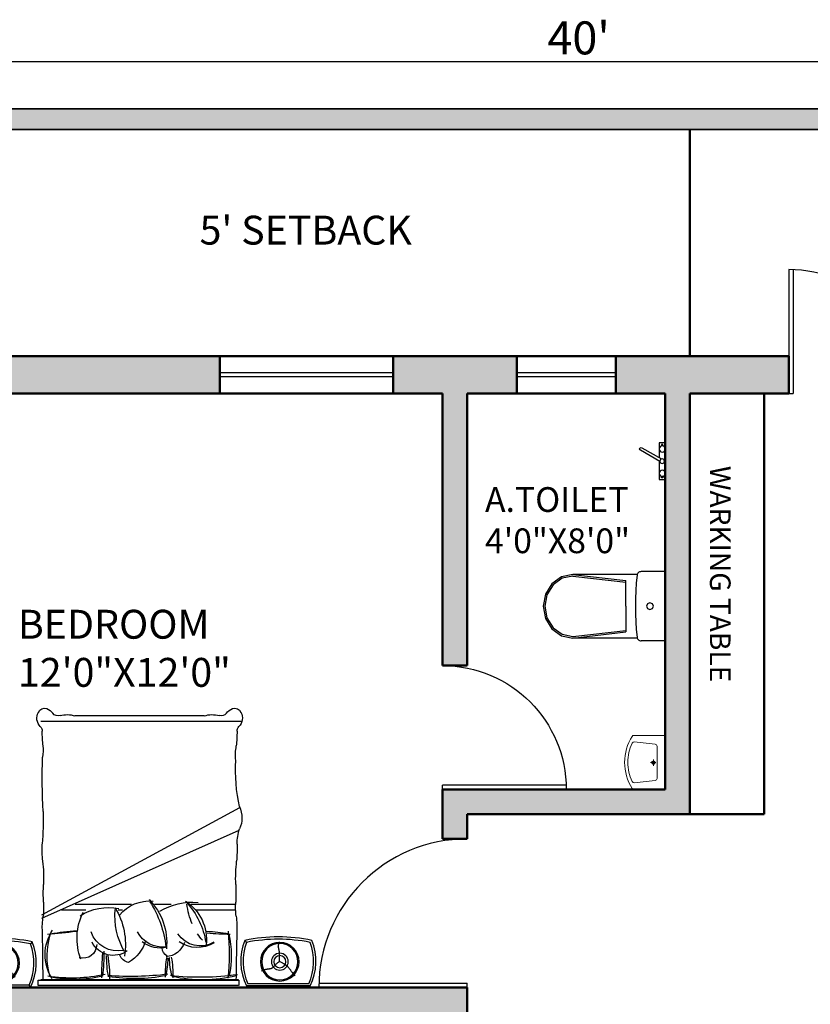
# Model space of a CAD drawing. Units: inches. Extents: x 3008 to 4088, y 1255 to 2137.
# Tile 19 of 30: x 3144 to 3336, y 1787 to 2026. Entities that reach past the tile are written whole.
import ezdxf

# ---------------------------------------------------------------- set-up
doc = ezdxf.new("R2010")
doc.units = ezdxf.units.IN
for name, color, linetype, lineweight in [('A-ANNO-DIMS', 2, 'Continuous', 18), ('A-ANNO-TEXT', 7, 'Continuous', 18), ('A-AREA-IDEN', 7, 'Continuous', 18), ('A-DOOR', 4, 'Continuous', 25), ('A-FLOR-FIXT', 8, 'Continuous', 18), ('A-FURN', 8, 'Continuous', 18), ('A-GLAZ', 4, 'Continuous', 25), ('A-WALL', 7, 'Continuous', 50), ('A-WALL-PATT', 8, 'Continuous', 13), ('C-PROP', 1, 'Continuous', 35), ('C-PROP-PATT', 9, 'Continuous', 13)]:
    doc.layers.add(name, color=color, linetype=linetype, lineweight=lineweight)
doc.layers.add('SANTEH', color=7, linetype='Continuous')
doc.layers.add('TEFRİŞ', color=11, linetype='Continuous')
doc.styles.get("Standard").update_dxf_attribs({"font": 'arial.ttf'})
doc.dimstyles.new('ISO-25', dxfattribs={"dimtxt": 8, "dimasz": 2.5, "dimexe": 1.25, "dimexo": 0.625, "dimtad": 1, "dimdec": 1, "dimlunit": 3, "dimtxsty": 'Standard', "dimcen": 2.5, "dimadec": 0, "dimazin": 0, "dimtfac": 1, "dimtdec": 1, "dimtmove": 0, "dimatfit": 3, "dimfxl": 1, "dimarcsym": 0})

# ---------------------------------------------------------------- blocks, each defined once
blk = doc.blocks.new('*D1')
at = {"layer": 'A-ANNO-DIMS', "color": 0, "lineweight": -2, "transparency": 16777216}
for p, q in [((3039.67, 2004.59), (3039.67, 2016.66)), ((3042.17, 2015.41), (3517.17, 2015.41)), ((3519.67, 2004.59), (3519.67, 2016.66))]:
    blk.add_line(p, q, dxfattribs=at)
at = {"layer": 'A-ANNO-DIMS', "color": 0, "transparency": 16777216}
for points in [[(3042.17, 2015.82), (3042.17, 2014.99), (3039.67, 2015.41)], [(3517.17, 2015.82), (3517.17, 2014.99), (3519.67, 2015.41)]]:
    blk.add_solid(points, dxfattribs=at)
at = {"layer": 'Defpoints', "color": 0, "transparency": 16777216}
for p in [(3519.67, 2015.41), (3039.67, 2003.97), (3519.67, 2003.97)]:
    blk.add_point(p, dxfattribs=at)
at = {"layer": 'A-ANNO-DIMS', "color": 0, "transparency": 16777216, "insert": (3279.67, 2020.12), "char_height": 8, "attachment_point": 5}
blk.add_mtext("40'", dxfattribs=at)
blk = doc.blocks.new('D2')
for p, q in [((1722.5, 1505.46), (1722.5, 1475.46)), ((1723.5, 1505.46), (1723.5, 1475.46)), ((1722.5, 1475.46), (1723.5, 1475.46))]:
    blk.add_line(p, q)
blk.add_arc((1722.5, 1475.46), 30, 0, 90)
blk = doc.blocks.new('D1')
for p, q in [((1805.96, 1500.36), (1805.96, 1464.36)), ((1806.96, 1500.36), (1806.96, 1464.36)), ((1805.96, 1464.36), (1806.96, 1464.36))]:
    blk.add_line(p, q)
blk.add_arc((1805.96, 1464.36), 36, 0, 90)
blk = doc.blocks.new('WC 2 Symb_109')
at = {"layer": 'SANTEH'}
for p, q in [((0, 0), (0, 380)), ((0, 380), (132.4, 380)), ((153.6, 364.9), (506.8, 364.9)), ((506.3, 364.9), (215.7, 330.9)), ((506.3, 356), (215.7, 322)), ((215.7, 190), (215.7, 330.9)), ((215.7, 190), (215.7, 49.1)), ((506.3, 24), (215.7, 58)), ((153.8, 15.1), (506.8, 15.1)), ((506.3, 15.1), (215.7, 49.1)), ((0, 0), (132.4, 0))]:
    blk.add_line(p, q, dxfattribs=at)
for points in [[(154.6, 360.1), (153.9, 364.1), (152.3, 367.9), (150.2, 371.3), (147.4, 374.3), (144.1, 376.7), (140.5, 378.5), (136.5, 379.6), (132.4, 380)], [(154.6, 19.7), (158.6, 62.1), (161.4, 104.7), (163.1, 147.3), (163.7, 189.9), (163.1, 232.5), (161.4, 275.1), (158.6, 317.7), (154.6, 360.1)], [(506.3, 24), (565.5, 36.6), (615.7, 72.6), (649.2, 126.5), (661, 190), (649.2, 253.5), (615.7, 307.4), (565.5, 343.4), (506.3, 356)], [(506.8, 15.1), (569.2, 28.4), (622.2, 66.3), (657.6, 123.1), (670, 190), (657.6, 256.9), (622.2, 313.7), (569.2, 351.6), (506.8, 364.9)], [(132.4, 0), (136.5, 0.4), (140.4, 1.5), (144.1, 3.2), (147.3, 5.6), (150.1, 8.6), (152.3, 12), (153.8, 15.7), (154.6, 19.7)]]:
    blk.add_lwpolyline(points, dxfattribs=at)
blk.add_lwpolyline([(83.6, 208.5), (70.4, 203.1), (64.9, 190), (70.4, 176.9), (83.6, 171.5), (96.8, 176.9), (102.2, 190), (96.8, 203.1)], close=True, dxfattribs=at)
blk = doc.blocks.new('Faucet - kit sink top')
at = {"layer": 'SANTEH'}
for p, q in [((-5.5, -0.75), (-5.5, -1.25)), ((-4.94278, -0.75), (-5.5, -0.75)), ((-5.5, -1.25), (-4.94278, -1.25)), ((-0.14775, -1.7441), (3.56698, -8.1782)), ((4.43301, -7.6782), (0.71828, -1.2441)), ((4.94278, -0.75), (5.5, -0.75)), ((5.5, -1.25), (4.94278, -1.25)), ((5.5, -0.75), (5.5, -1.25))]:
    blk.add_line(p, q, dxfattribs=at)
blk.add_lwpolyline([(-0.00587, -2), (-6, -2), (-6, 0), (6, 0), (6, -2), (1.15195, -2)], dxfattribs=at)
for centre, radius in [((-4, -1), 1), ((4, -1), 1), ((0, -1), 0.75)]:
    blk.add_circle(centre, radius, dxfattribs=at)
blk.add_arc((4, -7.9282), 0.5, 210, 30, dxfattribs=at)
blk = doc.blocks.new('A$C2EBB240D')
for p, q in [((480, 375.8), (20, 375.8)), ((0, 355.8), (0, 86.6)), ((60.8, 89.8), (82.3, 282.2)), ((250, 300), (102.1, 300)), ((250, 300), (397.9, 300)), ((439.2, 89.8), (417.7, 282.2)), ((500, 355.8), (500, 86.6))]:
    blk.add_line(p, q)
for points in [[(247.3, 238.5), (247.3, 288.9)], [(275.2, 266.4), (219.4, 266.4)]]:
    blk.add_lwpolyline(points)
for centre, radius, start, end in [((20, 355.8), 20, 90, 180), ((480, 355.8), 20, 0, 90), ((102.1, 280), 20, 90, 173.64284), ((247.3, 266.4), 16.7, 90, 270), ((247.3, 266.4), 10, 90, 270), ((247.3, 266.4), 16.7, 270, 90), ((247.3, 266.4), 10, 270, 90), ((397.9, 280), 20, 6.35716, 90), ((20, 86.6), 20, 180, 237.68921), ((250, 450.3), 450.3, 237.68921, 270), ((80.7, 87.6), 20, 173.64284, 244.97956), ((250, 450.3), 420.3, 244.97956, 270), ((250, 450.3), 450.3, 270, 302.31079), ((250, 450.3), 420.3, 270, 295.02044), ((419.3, 87.6), 20, 295.02044, 6.35716), ((480, 86.6), 20, 302.31079, 0)]:
    blk.add_arc(centre, radius, start, end)
blk = doc.blocks.new('BED')
at = {"layer": 'TEFRİŞ'}
for p, q in [((2114.88, 1835.66), (2129.12, 1835.66)), ((2115.2, 1835.15), (2128.8, 1835.15)), ((2130.81, 1834.34), (2130.81, 1835.55)), ((2175.56, 1834.34), (2130.81, 1834.34)), ((2130.91, 1835.55), (2175.56, 1835.55)), ((2175, 1834.19), (2130.91, 1834.19)), ((2175.56, 1835.55), (2175.56, 1834.34)), ((2177.29, 1835.98), (2177.61, 1835.47)), ((2177.29, 1835.98), (2191.52, 1835.98)), ((2177.61, 1835.47), (2191.2, 1835.47)), ((2191.2, 1835.47), (2191.52, 1835.98)), ((2118.49, 1833.2), (2118.34, 1833.38)), ((2118.49, 1833.2), (2118.34, 1833.38)), ((2118.63, 1833.03), (2118.49, 1833.2)), ((2118.63, 1833.03), (2118.49, 1833.2)), ((2118.75, 1832.88), (2118.63, 1833.03)), ((2118.75, 1832.88), (2118.63, 1833.03)), ((2118.86, 1832.74), (2118.75, 1832.88)), ((2118.86, 1832.74), (2118.75, 1832.88)), ((2118.95, 1832.61), (2118.86, 1832.74)), ((2118.95, 1832.61), (2118.86, 1832.74)), ((2119.04, 1832.48), (2118.95, 1832.61)), ((2119.04, 1832.48), (2118.95, 1832.61)), ((2119.12, 1832.37), (2119.04, 1832.48)), ((2119.12, 1832.37), (2119.04, 1832.48)), ((2119.19, 1832.26), (2119.12, 1832.37)), ((2119.19, 1832.26), (2119.12, 1832.37)), ((2119.26, 1832.16), (2119.19, 1832.26)), ((2119.26, 1832.16), (2119.19, 1832.26)), ((2119.32, 1832.06), (2119.26, 1832.16)), ((2119.32, 1832.06), (2119.26, 1832.16)), ((2119.39, 1831.97), (2119.32, 1832.06)), ((2119.39, 1831.97), (2119.32, 1832.06)), ((2119.45, 1831.89), (2119.39, 1831.97)), ((2119.45, 1831.89), (2119.39, 1831.97)), ((2119.51, 1831.81), (2119.45, 1831.89)), ((2119.51, 1831.81), (2119.45, 1831.89)), ((2119.57, 1831.73), (2119.51, 1831.81)), ((2119.57, 1831.73), (2119.51, 1831.81)), ((2119.63, 1831.65), (2119.57, 1831.73)), ((2119.63, 1831.65), (2119.57, 1831.73)), ((2119.69, 1831.58), (2119.63, 1831.65)), ((2119.69, 1831.58), (2119.63, 1831.65)), ((2123.27, 1831.58), (2123.34, 1831.63)), ((2123.27, 1831.58), (2123.34, 1831.63)), ((2123.34, 1831.63), (2123.41, 1831.67)), ((2123.34, 1831.63), (2123.41, 1831.67)), ((2123.41, 1831.67), (2123.48, 1831.71)), ((2123.41, 1831.67), (2123.48, 1831.71)), ((2123.48, 1831.71), (2123.55, 1831.74)), ((2123.48, 1831.71), (2123.55, 1831.74)), ((2123.55, 1831.74), (2123.62, 1831.77)), ((2123.55, 1831.74), (2123.62, 1831.77)), ((2123.62, 1831.77), (2123.69, 1831.8)), ((2123.62, 1831.77), (2123.69, 1831.8)), ((2123.69, 1831.8), (2123.77, 1831.82)), ((2123.69, 1831.8), (2123.77, 1831.82)), ((2123.77, 1831.82), (2123.84, 1831.84)), ((2123.77, 1831.82), (2123.84, 1831.84)), ((2123.84, 1831.84), (2123.91, 1831.86)), ((2123.84, 1831.84), (2123.91, 1831.86)), ((2123.91, 1831.86), (2123.98, 1831.87)), ((2123.91, 1831.86), (2123.98, 1831.87)), ((2123.98, 1831.87), (2124.06, 1831.89)), ((2123.98, 1831.87), (2124.06, 1831.89)), ((2124.06, 1831.89), (2124.13, 1831.9)), ((2124.06, 1831.89), (2124.13, 1831.9)), ((2124.13, 1831.9), (2124.2, 1831.91)), ((2124.13, 1831.9), (2124.2, 1831.91)), ((2124.2, 1831.91), (2124.27, 1831.91)), ((2124.2, 1831.91), (2124.27, 1831.91)), ((2124.27, 1831.91), (2124.35, 1831.92)), ((2124.27, 1831.91), (2124.35, 1831.92)), ((2124.35, 1831.92), (2124.42, 1831.93)), ((2124.35, 1831.92), (2124.42, 1831.93)), ((2124.42, 1831.93), (2124.49, 1831.94)), ((2124.42, 1831.93), (2124.49, 1831.94)), ((2124.49, 1831.94), (2124.56, 1831.95)), ((2124.49, 1831.94), (2124.56, 1831.95)), ((2124.56, 1831.95), (2124.64, 1831.96)), ((2124.56, 1831.95), (2124.64, 1831.96)), ((2124.64, 1831.96), (2124.71, 1831.98)), ((2124.64, 1831.96), (2124.71, 1831.98)), ((2124.71, 1831.98), (2124.79, 1831.99)), ((2124.71, 1831.98), (2124.79, 1831.99)), ((2124.79, 1831.99), (2124.87, 1832.01)), ((2124.79, 1831.99), (2124.87, 1832.01)), ((2124.87, 1832.01), (2124.96, 1832.03)), ((2124.87, 1832.01), (2124.96, 1832.03)), ((2124.96, 1832.03), (2125.05, 1832.05)), ((2124.96, 1832.03), (2125.05, 1832.05)), ((2125.05, 1832.05), (2125.14, 1832.08)), ((2125.05, 1832.05), (2125.14, 1832.08)), ((2125.14, 1832.08), (2125.23, 1832.11)), ((2125.14, 1832.08), (2125.23, 1832.11)), ((2125.23, 1832.11), (2125.33, 1832.14)), ((2125.23, 1832.11), (2125.33, 1832.14)), ((2125.33, 1832.14), (2125.42, 1832.17)), ((2125.33, 1832.14), (2125.42, 1832.17)), ((2125.42, 1832.17), (2125.52, 1832.21)), ((2125.42, 1832.17), (2125.52, 1832.21)), ((2125.52, 1832.21), (2125.6, 1832.25)), ((2125.52, 1832.21), (2125.6, 1832.25)), ((2125.6, 1832.25), (2125.68, 1832.3)), ((2125.6, 1832.25), (2125.68, 1832.3)), ((2125.68, 1832.3), (2125.75, 1832.35)), ((2125.68, 1832.3), (2125.75, 1832.35)), ((2180.9, 1833.52), (2180.75, 1833.7)), ((2180.9, 1833.52), (2180.75, 1833.7)), ((2181.04, 1833.35), (2180.9, 1833.52)), ((2181.04, 1833.35), (2180.9, 1833.52)), ((2181.16, 1833.2), (2181.04, 1833.35)), ((2181.16, 1833.2), (2181.04, 1833.35)), ((2181.26, 1833.06), (2181.16, 1833.2)), ((2181.26, 1833.06), (2181.16, 1833.2)), ((2181.36, 1832.93), (2181.26, 1833.06)), ((2181.36, 1832.93), (2181.26, 1833.06)), ((2181.44, 1832.8), (2181.36, 1832.93)), ((2181.44, 1832.8), (2181.36, 1832.93)), ((2181.52, 1832.69), (2181.44, 1832.8)), ((2181.52, 1832.69), (2181.44, 1832.8)), ((2181.59, 1832.58), (2181.52, 1832.69)), ((2181.59, 1832.58), (2181.52, 1832.69)), ((2181.66, 1832.48), (2181.59, 1832.58)), ((2181.66, 1832.48), (2181.59, 1832.58)), ((2181.73, 1832.38), (2181.66, 1832.48)), ((2181.73, 1832.38), (2181.66, 1832.48)), ((2181.79, 1832.29), (2181.73, 1832.38)), ((2181.79, 1832.29), (2181.73, 1832.38)), ((2181.85, 1832.21), (2181.79, 1832.29)), ((2181.85, 1832.21), (2181.79, 1832.29)), ((2181.92, 1832.13), (2181.85, 1832.21)), ((2181.92, 1832.13), (2181.85, 1832.21)), ((2181.97, 1832.05), (2181.92, 1832.13)), ((2181.97, 1832.05), (2181.92, 1832.13)), ((2182.03, 1831.97), (2181.97, 1832.05)), ((2182.03, 1831.97), (2181.97, 1832.05)), ((2182.09, 1831.9), (2182.03, 1831.97)), ((2182.09, 1831.9), (2182.03, 1831.97)), ((2182.15, 1831.83), (2182.09, 1831.9)), ((2182.15, 1831.83), (2182.09, 1831.9)), ((2182.21, 1831.76), (2182.15, 1831.83)), ((2182.21, 1831.76), (2182.15, 1831.83)), ((2182.27, 1831.7), (2182.21, 1831.76)), ((2182.27, 1831.7), (2182.21, 1831.76)), ((2182.33, 1831.63), (2182.27, 1831.7)), ((2182.33, 1831.63), (2182.27, 1831.7)), ((2182.4, 1831.57), (2182.33, 1831.63)), ((2182.4, 1831.57), (2182.33, 1831.63)), ((2185.35, 1831.58), (2185.42, 1831.65)), ((2185.35, 1831.58), (2185.42, 1831.65)), ((2185.42, 1831.65), (2185.48, 1831.72)), ((2185.42, 1831.65), (2185.48, 1831.72)), ((2185.48, 1831.72), (2185.55, 1831.78)), ((2185.48, 1831.72), (2185.55, 1831.78)), ((2185.55, 1831.78), (2185.61, 1831.84)), ((2185.55, 1831.78), (2185.61, 1831.84)), ((2185.61, 1831.84), (2185.68, 1831.9)), ((2185.61, 1831.84), (2185.68, 1831.9)), ((2185.68, 1831.9), (2185.75, 1831.95)), ((2185.68, 1831.9), (2185.75, 1831.95)), ((2185.75, 1831.95), (2185.82, 1831.99)), ((2185.75, 1831.95), (2185.82, 1831.99)), ((2185.82, 1831.99), (2185.89, 1832.03)), ((2185.82, 1831.99), (2185.89, 1832.03)), ((2185.89, 1832.03), (2185.96, 1832.06)), ((2185.89, 1832.03), (2185.96, 1832.06)), ((2185.96, 1832.06), (2186.03, 1832.09)), ((2185.96, 1832.06), (2186.03, 1832.09)), ((2186.03, 1832.09), (2186.1, 1832.12)), ((2186.03, 1832.09), (2186.1, 1832.12)), ((2186.1, 1832.12), (2186.17, 1832.14)), ((2186.1, 1832.12), (2186.17, 1832.14)), ((2186.17, 1832.14), (2186.24, 1832.16)), ((2186.17, 1832.14), (2186.24, 1832.16)), ((2186.24, 1832.16), (2186.32, 1832.18)), ((2186.24, 1832.16), (2186.32, 1832.18)), ((2186.32, 1832.18), (2186.39, 1832.19)), ((2186.32, 1832.18), (2186.39, 1832.19)), ((2186.39, 1832.19), (2186.46, 1832.21)), ((2186.39, 1832.19), (2186.46, 1832.21)), ((2186.46, 1832.21), (2186.53, 1832.22)), ((2186.46, 1832.21), (2186.53, 1832.22)), ((2186.53, 1832.22), (2186.61, 1832.23)), ((2186.53, 1832.22), (2186.61, 1832.23)), ((2186.61, 1832.23), (2186.68, 1832.23)), ((2186.61, 1832.23), (2186.68, 1832.23)), ((2186.68, 1832.23), (2186.75, 1832.24)), ((2186.68, 1832.23), (2186.75, 1832.24)), ((2186.75, 1832.24), (2186.82, 1832.25)), ((2186.75, 1832.24), (2186.82, 1832.25)), ((2186.82, 1832.25), (2186.9, 1832.26)), ((2186.82, 1832.25), (2186.9, 1832.26)), ((2186.9, 1832.26), (2186.97, 1832.27)), ((2186.9, 1832.26), (2186.97, 1832.27)), ((2186.97, 1832.27), (2187.04, 1832.28)), ((2186.97, 1832.27), (2187.04, 1832.28)), ((2187.04, 1832.28), (2187.12, 1832.3)), ((2187.04, 1832.28), (2187.12, 1832.3)), ((2187.12, 1832.3), (2187.2, 1832.31)), ((2187.12, 1832.3), (2187.2, 1832.31)), ((2187.2, 1832.31), (2187.28, 1832.33)), ((2187.2, 1832.31), (2187.28, 1832.33)), ((2187.28, 1832.33), (2187.36, 1832.35)), ((2187.28, 1832.33), (2187.36, 1832.35)), ((2187.36, 1832.35), (2187.45, 1832.37)), ((2187.36, 1832.35), (2187.45, 1832.37)), ((2187.45, 1832.37), (2187.54, 1832.4)), ((2187.45, 1832.37), (2187.54, 1832.4)), ((2187.54, 1832.4), (2187.64, 1832.43)), ((2187.54, 1832.4), (2187.64, 1832.43)), ((2187.64, 1832.43), (2187.74, 1832.46)), ((2187.64, 1832.43), (2187.74, 1832.46)), ((2187.74, 1832.46), (2187.83, 1832.49)), ((2187.74, 1832.46), (2187.83, 1832.49)), ((2187.83, 1832.49), (2187.92, 1832.53)), ((2187.83, 1832.49), (2187.92, 1832.53)), ((2187.92, 1832.53), (2188.01, 1832.57)), ((2187.92, 1832.53), (2188.01, 1832.57)), ((2188.01, 1832.57), (2188.09, 1832.62)), ((2188.01, 1832.57), (2188.09, 1832.62)), ((2188.09, 1832.62), (2188.15, 1832.67)), ((2188.09, 1832.62), (2188.15, 1832.67)), ((2119.75, 1831.51), (2119.69, 1831.58)), ((2119.75, 1831.51), (2119.69, 1831.58)), ((2119.81, 1831.44), (2119.75, 1831.51)), ((2119.81, 1831.44), (2119.75, 1831.51)), ((2119.87, 1831.38), (2119.81, 1831.44)), ((2119.87, 1831.38), (2119.81, 1831.44)), ((2119.93, 1831.31), (2119.87, 1831.38)), ((2119.93, 1831.31), (2119.87, 1831.38)), ((2119.99, 1831.25), (2119.93, 1831.31)), ((2119.99, 1831.25), (2119.93, 1831.31)), ((2120.05, 1831.2), (2119.99, 1831.25)), ((2120.05, 1831.2), (2119.99, 1831.25)), ((2120.12, 1831.14), (2120.05, 1831.2)), ((2120.12, 1831.14), (2120.05, 1831.2)), ((2120.18, 1831.09), (2120.12, 1831.14)), ((2120.18, 1831.09), (2120.12, 1831.14)), ((2120.25, 1831.04), (2120.18, 1831.09)), ((2120.25, 1831.04), (2120.18, 1831.09)), ((2120.32, 1830.99), (2120.25, 1831.04)), ((2120.32, 1830.99), (2120.25, 1831.04)), ((2120.39, 1830.94), (2120.32, 1830.99)), ((2120.39, 1830.94), (2120.32, 1830.99)), ((2120.47, 1830.9), (2120.39, 1830.94)), ((2120.47, 1830.9), (2120.39, 1830.94)), ((2120.54, 1830.85), (2120.47, 1830.9)), ((2120.54, 1830.85), (2120.47, 1830.9)), ((2120.62, 1830.8), (2120.54, 1830.85)), ((2120.62, 1830.8), (2120.54, 1830.85)), ((2120.7, 1830.75), (2120.62, 1830.8)), ((2120.7, 1830.75), (2120.62, 1830.8)), ((2120.79, 1830.7), (2120.7, 1830.75)), ((2120.79, 1830.7), (2120.7, 1830.75)), ((2120.88, 1830.65), (2120.79, 1830.7)), ((2120.88, 1830.65), (2120.79, 1830.7)), ((2120.98, 1830.59), (2120.88, 1830.65)), ((2120.98, 1830.59), (2120.88, 1830.65)), ((2121.09, 1830.52), (2120.98, 1830.59)), ((2121.09, 1830.52), (2120.98, 1830.59)), ((2121.21, 1830.45), (2121.09, 1830.52)), ((2121.21, 1830.45), (2121.09, 1830.52)), ((2121.34, 1830.38), (2121.21, 1830.45)), ((2121.34, 1830.38), (2121.21, 1830.45)), ((2121.49, 1830.29), (2121.34, 1830.38)), ((2121.49, 1830.29), (2121.34, 1830.38)), ((2121.66, 1830.21), (2121.49, 1830.29)), ((2121.66, 1830.21), (2121.49, 1830.29)), ((2121.66, 1830.18), (2121.87, 1830.29)), ((2121.66, 1830.18), (2121.87, 1830.29)), ((2121.85, 1830.11), (2121.66, 1830.21)), ((2121.85, 1830.11), (2121.66, 1830.21)), ((2121.74, 1829.99), (2121.73, 1829.83)), ((2121.74, 1829.99), (2121.73, 1829.83)), ((2121.73, 1829.83), (2121.73, 1829.69)), ((2121.73, 1829.83), (2121.73, 1829.69)), ((2121.73, 1829.69), (2121.73, 1829.57)), ((2121.73, 1829.69), (2121.73, 1829.57)), ((2121.73, 1829.57), (2121.73, 1829.45)), ((2121.73, 1829.57), (2121.73, 1829.45)), ((2121.73, 1829.45), (2121.74, 1829.35)), ((2121.73, 1829.45), (2121.74, 1829.35)), ((2121.76, 1830.38), (2121.74, 1830.17)), ((2121.76, 1830.38), (2121.74, 1830.17)), ((2121.74, 1830.17), (2121.74, 1829.99)), ((2121.74, 1830.17), (2121.74, 1829.99)), ((2121.87, 1830.29), (2122.04, 1830.4)), ((2121.87, 1830.29), (2122.04, 1830.4)), ((2122.04, 1830.4), (2122.2, 1830.51)), ((2122.04, 1830.4), (2122.2, 1830.51)), ((2122.2, 1830.51), (2122.33, 1830.61)), ((2122.2, 1830.51), (2122.33, 1830.61)), ((2122.33, 1830.61), (2122.45, 1830.72)), ((2122.33, 1830.61), (2122.45, 1830.72)), ((2122.45, 1830.72), (2122.55, 1830.82)), ((2122.45, 1830.72), (2122.55, 1830.82)), ((2122.55, 1830.82), (2122.64, 1830.91)), ((2122.55, 1830.82), (2122.64, 1830.91)), ((2122.64, 1830.91), (2122.72, 1831.01)), ((2122.64, 1830.91), (2122.72, 1831.01)), ((2122.72, 1831.01), (2122.8, 1831.09)), ((2122.72, 1831.01), (2122.8, 1831.09)), ((2122.8, 1831.09), (2122.87, 1831.18)), ((2122.8, 1831.09), (2122.87, 1831.18)), ((2122.87, 1831.18), (2122.94, 1831.26)), ((2122.87, 1831.18), (2122.94, 1831.26)), ((2122.94, 1831.26), (2123.01, 1831.33)), ((2122.94, 1831.26), (2123.01, 1831.33)), ((2123.01, 1831.33), (2123.08, 1831.4)), ((2123.01, 1831.33), (2123.08, 1831.4)), ((2123.08, 1831.4), (2123.14, 1831.46)), ((2123.08, 1831.4), (2123.14, 1831.46)), ((2123.14, 1831.46), (2123.21, 1831.52)), ((2123.14, 1831.46), (2123.21, 1831.52)), ((2123.21, 1831.52), (2123.27, 1831.58)), ((2123.21, 1831.52), (2123.27, 1831.58)), ((2182.46, 1831.52), (2182.4, 1831.57)), ((2182.46, 1831.52), (2182.4, 1831.57)), ((2182.52, 1831.46), (2182.46, 1831.52)), ((2182.52, 1831.46), (2182.46, 1831.52)), ((2182.59, 1831.41), (2182.52, 1831.46)), ((2182.59, 1831.41), (2182.52, 1831.46)), ((2182.66, 1831.36), (2182.59, 1831.41)), ((2182.66, 1831.36), (2182.59, 1831.41)), ((2182.73, 1831.31), (2182.66, 1831.36)), ((2182.73, 1831.31), (2182.66, 1831.36)), ((2182.8, 1831.26), (2182.73, 1831.31)), ((2182.8, 1831.26), (2182.73, 1831.31)), ((2182.87, 1831.22), (2182.8, 1831.26)), ((2182.87, 1831.22), (2182.8, 1831.26)), ((2182.95, 1831.17), (2182.87, 1831.22)), ((2182.95, 1831.17), (2182.87, 1831.22)), ((2183.03, 1831.12), (2182.95, 1831.17)), ((2183.03, 1831.12), (2182.95, 1831.17)), ((2183.11, 1831.07), (2183.03, 1831.12)), ((2183.11, 1831.07), (2183.03, 1831.12)), ((2183.2, 1831.02), (2183.11, 1831.07)), ((2183.2, 1831.02), (2183.11, 1831.07)), ((2183.29, 1830.97), (2183.2, 1831.02)), ((2183.29, 1830.97), (2183.2, 1831.02)), ((2183.39, 1830.91), (2183.29, 1830.97)), ((2183.39, 1830.91), (2183.29, 1830.97)), ((2183.49, 1830.84), (2183.39, 1830.91)), ((2183.49, 1830.84), (2183.39, 1830.91)), ((2183.61, 1830.77), (2183.49, 1830.84)), ((2183.61, 1830.77), (2183.49, 1830.84)), ((2183.75, 1830.7), (2183.61, 1830.77)), ((2183.75, 1830.7), (2183.61, 1830.77)), ((2183.9, 1830.61), (2183.75, 1830.7)), ((2183.9, 1830.61), (2183.75, 1830.7)), ((2184.06, 1830.53), (2183.9, 1830.61)), ((2184.06, 1830.53), (2183.9, 1830.61)), ((2184.25, 1830.43), (2184.06, 1830.53)), ((2184.25, 1830.43), (2184.06, 1830.53)), ((2184.07, 1830.5), (2184.27, 1830.61)), ((2184.07, 1830.5), (2184.27, 1830.61)), ((2184.15, 1830.49), (2184.14, 1830.31)), ((2184.15, 1830.49), (2184.14, 1830.31)), ((2184.14, 1830.31), (2184.14, 1830.15)), ((2184.14, 1830.31), (2184.14, 1830.15)), ((2184.14, 1830.15), (2184.14, 1830.01)), ((2184.14, 1830.15), (2184.14, 1830.01)), ((2184.14, 1830.01), (2184.14, 1829.89)), ((2184.14, 1830.01), (2184.14, 1829.89)), ((2184.14, 1829.89), (2184.14, 1829.77)), ((2184.14, 1829.89), (2184.14, 1829.77)), ((2184.14, 1829.77), (2184.14, 1829.67)), ((2184.14, 1829.77), (2184.14, 1829.67)), ((2184.14, 1829.67), (2184.15, 1829.57)), ((2184.14, 1829.67), (2184.15, 1829.57)), ((2184.17, 1830.7), (2184.15, 1830.49)), ((2184.17, 1830.7), (2184.15, 1830.49)), ((2184.15, 1829.57), (2184.15, 1829.48)), ((2184.15, 1829.57), (2184.15, 1829.48)), ((2184.15, 1829.48), (2184.15, 1829.38)), ((2184.15, 1829.48), (2184.15, 1829.38)), ((2184.27, 1830.61), (2184.45, 1830.72)), ((2184.27, 1830.61), (2184.45, 1830.72)), ((2184.45, 1830.72), (2184.6, 1830.83)), ((2184.45, 1830.72), (2184.6, 1830.83)), ((2184.6, 1830.83), (2184.74, 1830.93)), ((2184.6, 1830.83), (2184.74, 1830.93)), ((2184.74, 1830.93), (2184.85, 1831.04)), ((2184.74, 1830.93), (2184.85, 1831.04)), ((2184.85, 1831.04), (2184.95, 1831.14)), ((2184.85, 1831.04), (2184.95, 1831.14)), ((2184.95, 1831.14), (2185.05, 1831.23)), ((2184.95, 1831.14), (2185.05, 1831.23)), ((2185.05, 1831.23), (2185.13, 1831.33)), ((2185.05, 1831.23), (2185.13, 1831.33)), ((2185.13, 1831.33), (2185.21, 1831.41)), ((2185.13, 1831.33), (2185.21, 1831.41)), ((2185.21, 1831.41), (2185.28, 1831.5)), ((2185.21, 1831.41), (2185.28, 1831.5)), ((2185.28, 1831.5), (2185.35, 1831.58)), ((2185.28, 1831.5), (2185.35, 1831.58)), ((2121.74, 1828.89), (2121.73, 1828.8)), ((2121.74, 1828.89), (2121.73, 1828.8)), ((2121.73, 1828.8), (2121.73, 1828.72)), ((2121.73, 1828.8), (2121.73, 1828.72)), ((2121.73, 1828.72), (2121.73, 1828.64)), ((2121.73, 1828.72), (2121.73, 1828.64)), ((2121.73, 1828.64), (2121.73, 1828.56)), ((2121.73, 1828.64), (2121.73, 1828.56)), ((2121.73, 1828.56), (2121.73, 1828.48)), ((2121.73, 1828.56), (2121.73, 1828.48)), ((2121.73, 1828.48), (2121.73, 1828.4)), ((2121.73, 1828.48), (2121.73, 1828.4)), ((2121.73, 1828.4), (2121.73, 1828.33)), ((2121.73, 1828.4), (2121.73, 1828.33)), ((2121.73, 1828.33), (2121.74, 1828.25)), ((2121.73, 1828.33), (2121.74, 1828.25)), ((2121.74, 1829.35), (2121.74, 1829.25)), ((2121.74, 1829.35), (2121.74, 1829.25)), ((2121.74, 1829.25), (2121.74, 1829.16)), ((2121.74, 1829.25), (2121.74, 1829.16)), ((2121.74, 1829.16), (2121.74, 1829.06)), ((2121.74, 1829.16), (2121.74, 1829.06)), ((2121.74, 1829.06), (2121.74, 1828.97)), ((2121.74, 1829.06), (2121.74, 1828.97)), ((2121.74, 1828.97), (2121.74, 1828.89)), ((2121.74, 1828.97), (2121.74, 1828.89)), ((2121.74, 1828.25), (2121.75, 1828.18)), ((2121.74, 1828.25), (2121.75, 1828.18)), ((2121.75, 1828.18), (2121.75, 1828.1)), ((2121.75, 1828.18), (2121.75, 1828.1)), ((2121.75, 1828.1), (2121.76, 1828.03)), ((2121.75, 1828.1), (2121.76, 1828.03)), ((2121.76, 1828.03), (2121.78, 1827.95)), ((2121.76, 1828.03), (2121.78, 1827.95)), ((2121.78, 1827.95), (2121.79, 1827.88)), ((2121.78, 1827.95), (2121.79, 1827.88)), ((2121.79, 1827.88), (2121.8, 1827.8)), ((2121.79, 1827.88), (2121.8, 1827.8)), ((2121.8, 1827.8), (2121.82, 1827.72)), ((2121.8, 1827.8), (2121.82, 1827.72)), ((2121.82, 1827.72), (2121.84, 1827.65)), ((2121.82, 1827.72), (2121.84, 1827.65)), ((2121.84, 1827.65), (2121.85, 1827.57)), ((2121.84, 1827.65), (2121.85, 1827.57)), ((2121.85, 1827.57), (2121.87, 1827.49)), ((2121.85, 1827.57), (2121.87, 1827.49)), ((2121.87, 1827.49), (2121.89, 1827.41)), ((2121.87, 1827.49), (2121.89, 1827.41)), ((2121.89, 1827.41), (2121.91, 1827.33)), ((2121.89, 1827.41), (2121.91, 1827.33)), ((2121.91, 1827.33), (2121.93, 1827.26)), ((2121.91, 1827.33), (2121.93, 1827.26)), ((2121.93, 1827.26), (2121.95, 1827.18)), ((2121.93, 1827.26), (2121.95, 1827.18)), ((2184.14, 1829.04), (2184.13, 1828.96)), ((2184.14, 1829.04), (2184.13, 1828.96)), ((2184.13, 1828.96), (2184.13, 1828.88)), ((2184.13, 1828.96), (2184.13, 1828.88)), ((2184.13, 1828.88), (2184.13, 1828.8)), ((2184.13, 1828.88), (2184.13, 1828.8)), ((2184.13, 1828.8), (2184.14, 1828.72)), ((2184.13, 1828.8), (2184.14, 1828.72)), ((2184.15, 1829.38), (2184.14, 1829.29)), ((2184.15, 1829.38), (2184.14, 1829.29)), ((2184.14, 1829.29), (2184.14, 1829.21)), ((2184.14, 1829.29), (2184.14, 1829.21)), ((2184.14, 1829.21), (2184.14, 1829.12)), ((2184.14, 1829.21), (2184.14, 1829.12)), ((2184.14, 1829.12), (2184.14, 1829.04)), ((2184.14, 1829.12), (2184.14, 1829.04)), ((2184.14, 1828.72), (2184.14, 1828.65)), ((2184.14, 1828.72), (2184.14, 1828.65)), ((2184.14, 1828.65), (2184.15, 1828.57)), ((2184.14, 1828.65), (2184.15, 1828.57)), ((2184.15, 1828.57), (2184.15, 1828.5)), ((2184.15, 1828.57), (2184.15, 1828.5)), ((2184.15, 1828.5), (2184.16, 1828.42)), ((2184.15, 1828.5), (2184.16, 1828.42)), ((2184.16, 1828.42), (2184.17, 1828.35)), ((2184.16, 1828.42), (2184.17, 1828.35)), ((2184.17, 1828.35), (2184.18, 1828.27)), ((2184.17, 1828.35), (2184.18, 1828.27)), ((2184.18, 1828.27), (2184.19, 1828.2)), ((2184.18, 1828.27), (2184.19, 1828.2)), ((2184.19, 1828.2), (2184.21, 1828.12)), ((2184.19, 1828.2), (2184.21, 1828.12)), ((2184.21, 1828.12), (2184.22, 1828.04)), ((2184.21, 1828.12), (2184.22, 1828.04)), ((2184.22, 1828.04), (2184.24, 1827.97)), ((2184.22, 1828.04), (2184.24, 1827.97)), ((2184.24, 1827.97), (2184.26, 1827.89)), ((2184.24, 1827.97), (2184.26, 1827.89)), ((2184.26, 1827.89), (2184.28, 1827.81)), ((2184.26, 1827.89), (2184.28, 1827.81)), ((2184.28, 1827.81), (2184.3, 1827.73)), ((2184.28, 1827.81), (2184.3, 1827.73)), ((2184.3, 1827.73), (2184.32, 1827.65)), ((2184.3, 1827.73), (2184.32, 1827.65)), ((2184.32, 1827.65), (2184.34, 1827.58)), ((2184.32, 1827.65), (2184.34, 1827.58)), ((2184.34, 1827.58), (2184.36, 1827.5)), ((2184.34, 1827.58), (2184.36, 1827.5)), ((2184.36, 1827.5), (2184.38, 1827.41)), ((2184.36, 1827.5), (2184.38, 1827.41)), ((2184.38, 1827.41), (2184.4, 1827.33)), ((2184.38, 1827.41), (2184.4, 1827.33)), ((2184.4, 1827.33), (2184.41, 1827.25)), ((2184.4, 1827.33), (2184.41, 1827.25)), ((2184.41, 1827.25), (2184.41, 1827.16)), ((2184.41, 1827.25), (2184.41, 1827.16)), ((2121.78, 1825.93), (2121.74, 1825.8)), ((2121.78, 1825.93), (2121.74, 1825.8)), ((2121.83, 1826.06), (2121.78, 1825.93)), ((2121.83, 1826.06), (2121.78, 1825.93)), ((2121.87, 1826.19), (2121.83, 1826.06)), ((2121.87, 1826.19), (2121.83, 1826.06)), ((2121.91, 1826.31), (2121.87, 1826.19)), ((2121.91, 1826.31), (2121.87, 1826.19)), ((2121.95, 1826.42), (2121.91, 1826.31)), ((2121.95, 1826.42), (2121.91, 1826.31)), ((2121.95, 1827.18), (2121.97, 1827.09)), ((2121.95, 1827.18), (2121.97, 1827.09)), ((2121.97, 1826.54), (2121.95, 1826.42)), ((2121.97, 1826.54), (2121.95, 1826.42)), ((2121.97, 1827.09), (2121.99, 1827.01)), ((2121.97, 1827.09), (2121.99, 1827.01)), ((2121.99, 1826.64), (2121.97, 1826.54)), ((2121.99, 1826.64), (2121.97, 1826.54)), ((2121.99, 1827.01), (2122, 1826.93)), ((2121.99, 1827.01), (2122, 1826.93)), ((2122, 1826.74), (2121.99, 1826.64)), ((2122, 1826.74), (2121.99, 1826.64)), ((2122, 1826.93), (2122.01, 1826.84)), ((2122, 1826.93), (2122.01, 1826.84)), ((2122.01, 1826.84), (2122, 1826.74)), ((2122.01, 1826.84), (2122, 1826.74)), ((2129.46, 1825.49), (2129.09, 1825.93)), ((2176.94, 1825.81), (2177.31, 1826.25)), ((2184.19, 1826.25), (2184.14, 1826.12)), ((2184.19, 1826.25), (2184.14, 1826.12)), ((2184.23, 1826.38), (2184.19, 1826.25)), ((2184.23, 1826.38), (2184.19, 1826.25)), ((2184.28, 1826.51), (2184.23, 1826.38)), ((2184.28, 1826.51), (2184.23, 1826.38)), ((2184.32, 1826.63), (2184.28, 1826.51)), ((2184.32, 1826.63), (2184.28, 1826.51)), ((2184.35, 1826.74), (2184.32, 1826.63)), ((2184.35, 1826.74), (2184.32, 1826.63)), ((2184.38, 1826.86), (2184.35, 1826.74)), ((2184.38, 1826.86), (2184.35, 1826.74)), ((2184.4, 1826.96), (2184.38, 1826.86)), ((2184.4, 1826.96), (2184.38, 1826.86)), ((2184.41, 1827.06), (2184.4, 1826.96)), ((2184.41, 1827.06), (2184.4, 1826.96)), ((2184.41, 1827.16), (2184.41, 1827.06)), ((2184.41, 1827.16), (2184.41, 1827.06)), ((2191.87, 1825.81), (2191.5, 1826.25)), ((2174.77, 1819.77), (2130.6, 1795.83)), ((2174.77, 1820.53), (2130.76, 1800.91)), ((2140.43, 1818.69), (2131.53, 1818.69)), ((2157.71, 1818.69), (2156.77, 1818.69)), ((2170.41, 1818.69), (2164.92, 1818.69)), ((2141.43, 1817.4), (2131.53, 1817.4)), ((2149.62, 1817.4), (2145.88, 1817.4)), ((2167.36, 1817.4), (2154.77, 1817.4)), ((2175, 1776.57), (2130.11, 1776.57)), ((2138.52, 1775.41), (2167.39, 1775.41))]:
    blk.add_line(p, q, dxfattribs=at)
for centre, radius, start, end in [((2126, 1830.19), 12.39, 153.8162, 202.314), ((2126, 1830.19), 11.88, 155.3335, 201.0157), ((2118, 1830.19), 11.88, 338.9843, 24.6665), ((2118, 1830.19), 12.39, 337.686, 26.1838), ((2188.4, 1830.51), 12.39, 153.8162, 202.314), ((2188.4, 1830.51), 11.88, 155.3335, 201.0157), ((2180.41, 1830.51), 11.88, 338.9843, 24.6665), ((2180.41, 1830.51), 12.39, 337.686, 26.1838), ((2122, 1861.35), 36.63, 258.2443, 281.7557), ((2122, 1861.35), 36.12, 258.6773, 281.3227), ((2184.41, 1861.67), 36.63, 258.2443, 281.7557), ((2184.41, 1861.67), 36.12, 258.6773, 281.3227)]:
    blk.add_arc(centre, radius, start, end, dxfattribs=at)
at = {"layer": 'TEFRİŞ', "extrusion": (0, 0, -1)}
for centre, major_axis, ratio, start_param, end_param in [((2121.68, 1830.24), (-3.05, -3.05), 1, 3.926991, 10.210176), ((2121.68, 1830.24), (2.86, -2.86), 1, 5.497787, 11.780972), ((2121.68, 1830.24), (2.86, -2.86), 1, 5.497787, 11.780972), ((2139.43, 1773.84), (-42.35, 42.35), 1, 0.646251, 0.896949), ((2206.14, 1830.73), (-52.86, -52.86), 1, 0.767743, 0.83177), ((2138.85, 1803.05), (-22.1, 22.1), 1, 0.544604, 1.006234), ((2181.61, 1828.44), (-34.39, 34.39), 1, -0.888486, -0.672463), ((2164.51, 1832.79), (-13.41, 13.41), 1, -0.974476, -0.730892), ((2154.12, 1796.61), (-26.46, 26.46), 1, 0.596409, 0.940188), ((2183.72, 1833.22), (-17, 17), 1, -0.967105, -0.749712), ((2168.35, 1789.27), (-1.33, 44.62), 0.875277, -0.163954, 0.163954), ((2087.32, 1833.96), (-52.37, 52.37), 1, 2.358049, 2.431787), ((2167.6, 1797.72), (-0.51, 36.47), 0.865194, -0.185965, 0.185965), ((2164.15, 1828.7), (-6.99, 6.99), 1, 1.789136, 2.946702), ((2099.77, 1830.73), (-52.86, 52.86), 1, 2.311571, 2.373849), ((2184.09, 1830.56), (-3.05, -3.05), 1, 3.926991, 10.210176), ((2184.09, 1830.56), (2.86, -2.86), 1, 5.497787, 11.780972), ((2184.09, 1830.56), (2.86, -2.86), 1, 5.497787, 11.780972), ((2121.68, 1830.24), (1.33, -1.33), 1, 5.497787, 11.780972), ((2121.68, 1830.24), (1.33, -1.33), 1, 5.497787, 11.780972), ((2121.68, 1830.24), (0.952, -0.952), 1, 5.497787, 11.780972), ((2121.68, 1830.24), (0.952, -0.952), 1, 5.497787, 11.780972), ((2154.7, 1828.89), (-15.68, 15.68), 1, -1.00675, -0.580436), ((2127.6, 1828.81), (-13.23, 13.23), 1, 2.100388, 2.328052), ((2155, 1761.9), (-50.65, -50.65), 1, 2.239512, 2.426533), ((2172.01, 1828.66), (-17.93, 17.93), 1, -0.753394, -0.598744), ((2128.44, 1832.96), (-13.26, -13.26), 1, 3.889049, 4.127298), ((2134, 1828.8), (-18.62, 18.62), 1, 2.173461, 2.355043), ((2199.2, 1828.45), (-27.06, -27.06), 1, 0.770625, 0.917228), ((2156.76, 1828.98), (-11.9, -11.9), 1, 3.646453, 4.226155), ((2184.09, 1830.56), (1.33, -1.33), 1, 5.497787, 11.780972), ((2184.09, 1830.56), (1.33, -1.33), 1, 5.497787, 11.780972), ((2184.09, 1830.56), (0.952, -0.952), 1, 5.497787, 11.780972), ((2184.09, 1830.56), (0.952, -0.952), 1, 5.497787, 11.780972), ((2159.55, 1823.33), (-5.81, 5.81), 1, -0.516587, 0.256776), ((2154.84, 1827.75), (-1.93, 1.93), 1, 0.997904, 1.977819), ((2166.67, 1824.96), (-2.93, 3.91), 0.760601, -0.723751, 0.723751), ((2153.88, 1825.05), (-9.22, 9.22), 1, 1.994956, 2.818753), ((2675.38, 1815.09), (-384.79, -384.79), 1, 0.80103, 0.811711), ((2140.05, 1819.86), (-5.1, 5.1), 1, 0.238357, 1.390139), ((2139.42, 1820.79), (-4.21, -4.21), 1, 1.82161, 3.349145), ((2147.44, 1824.41), (-3.36, -3.36), 1, 1.11934, 2.270556), ((2160.6, 1825.98), (-9.68, -9.68), 1, 0.009196, 0.886853), ((2145.66, 1827.01), (-1.62, 1.62), 1, 1.310976, 2.284591), ((2148.35, 1820.65), (-4.63, -4.63), 1, 2.117602, 3.020837), ((2147.86, 1820.64), (-4.48, 4.48), 1, 0.665914, 1.867503), ((2172, 1826.44), (-11.23, 11.23), 1, -1.332486, -0.624868), ((2158.82, 1823.55), (-3.74, -3.74), 1, 1.730792, 3.47045), ((2141.71, 1819.83), (-11.86, 11.86), 1, 1.850844, 2.42862), ((2157.83, 1821.53), (-4.47, 4.47), 1, 0.576679, 2.021689), ((1630.53, 1815.09), (-384.79, 384.79), 1, 2.329881, 2.340562), ((2148.15, 1825.25), (-7.14, -7.14), 1, 6.061986, 7.190757), ((2154.93, 1828.48), (-11.96, 11.96), 1, -1.530302, -0.934407), ((2127.37, 1815.76), (-10.68, 10.68), 1, 1.657204, 1.779381), ((2170.68, 1829.67), (-16.79, 16.79), 1, -1.354718, -0.902276), ((2146.08, 1822.57), (-10.5, 10.5), 1, -0.951783, -0.716225), ((2132.43, 1774.09), (-35.41, -35.41), 1, 2.362911, 2.464592), ((2140.17, 1862.96), (-27.99, 27.99), 1, 3.983025, 4.107469), ((2165.73, 1860.69), (-26.41, -26.41), 1, 5.306413, 5.463767), ((2199.62, 1529.47), (-209.2, 209.2), 1, 0.675361, 0.697001), ((2159.82, 1822.57), (-10.5, -10.5), 1, 3.857817, 4.093375), ((2127.37, 1815.76), (-10.68, 10.68), 1, 1.94252, 2.248924), ((2111.06, 1818.12), (-14.48, 14.48), 1, 2.258605, 2.412359), ((2141.33, 1830.48), (-9.55, -9.55), 1, 4.941413, 5.601673), ((2150.79, 1825.18), (-6, 6), 1, 3.032122, 4.026148), ((2159.02, 1834.9), (-3.04, 16.53), 0.830169, 2.822117, 3.461068), ((2194.85, 1818.12), (-14.48, 14.48), 1, -0.841563, -0.687809), ((2169.92, 1815.01), (-27.2, -27.2), 1, 0.734393, 0.836404), ((2135.98, 1815.01), (-27.2, -27.2), 1, 3.875985, 3.977996), ((2098.24, 1811.68), (-23.54, -23.54), 1, 3.885834, 4.043401), ((2207.66, 1811.68), (-23.54, -23.54), 1, 0.668988, 0.826555), ((2189.03, 1803.74), (-40.91, -40.91), 1, 0.789771, 0.855756), ((2116.87, 1803.74), (-40.91, 40.91), 1, 2.285836, 2.351822), ((2122.14, 1803.63), (-6.39, -6.39), 1, 3.886359, 4.265474), ((2222.76, 1798.77), (-34.16, -34.16), 1, 0.743488, 0.893627), ((2135.02, 1798.41), (-3.45, 3.45), 1, -0.831635, -0.314979), ((2135.48, 1798), (-3.77, -3.77), 1, 0.329385, 0.820948), ((2148.06, 1790.38), (-0.75, 67.37), 0.394952, 1.480524, 1.661068), ((2127.76, 1790.23), (-1, 12.37), 0.296708, 1.141067, 2.000525), ((2118.49, 1784.2), (-9.24, -9.24), 1, 3.839645, 4.088086), ((2182.27, 1782.99), (-5.52, -5.52), 1, 0.671703, 0.993321), ((2162.12, 1778.86), (-21.85, 21.85), 1, -0.78611, -0.680117), ((2143.78, 1778.86), (-21.85, 21.85), 1, 2.250913, 2.356906), ((2132.72, 1775.92), (-1.91, -1.91), 1, 0.284117, 1.557111), ((2129.83, 1778.8), (-0.986, 0.986), 1, 2.330985, 3.163296), ((2176.08, 1778.8), (-0.986, 0.986), 1, 4.690686, 5.522997), ((2173.18, 1775.92), (-1.91, -1.91), 1, 3.155278, 4.428271), ((2131.79, 1775.28), (-1.11, 1.11), 1, 3.629269, 5.067473), ((2130.83, 1777), (-2.49, -2.49), 1, 4.590984, 5.084038), ((2134.73, 1774.06), (-0.964, -0.964), 1, 1.381176, 2.701227), ((2136.75, 1781.14), (-4.24, 4.24), 1, 3.62713, 4.188813), ((2169.16, 1781.14), (-4.24, 4.24), 1, 3.665169, 4.226852), ((2171.17, 1774.06), (-0.964, -0.964), 1, 2.011162, 3.331212), ((2175.07, 1777), (-2.49, 2.49), 1, 4.34074, 4.833793), ((2174.12, 1775.28), (-1.11, 1.11), 1, 2.786508, 4.224712)]:
    blk.add_ellipse(centre, major_axis=major_axis, ratio=ratio, start_param=start_param, end_param=end_param, dxfattribs=at)

msp = doc.modelspace()

# ---------------------------------------------------------------- hatches: boundary and pattern name
at = {"layer": 'A-WALL-PATT'}
h = msp.add_hatch(color=256, dxfattribs=at)
h.dxf.hatch_style = 1
h.paths.add_polyline_path([(3102.67, 1625.97), (3093.67, 1625.97), (3093.67, 1540.97), (3102.67, 1540.97)])
h.paths.add_polyline_path([(3102.67, 1784.97), (3252.67, 1784.97), (3252.67, 1790.97), (3102.67, 1790.97), (3102.67, 1892.97), (3093.67, 1892.97), (3093.67, 1667.97), (3102.67, 1667.97)])
h.paths.add_polyline_path([(3192.67, 1943.97), (3093.67, 1943.97), (3093.67, 1934.97), (3102.67, 1934.97), (3192.67, 1934.97)])
h.paths.add_polyline_path([(3264.67, 1943.97), (3234.67, 1943.97), (3234.67, 1934.97), (3246.67, 1934.97), (3246.67, 1868.97), (3252.67, 1868.97), (3252.67, 1934.97), (3264.67, 1934.97)])
h.paths.add_polyline_path([(3330.67, 1943.97), (3288.67, 1943.97), (3288.67, 1934.97), (3300.67, 1934.97), (3300.67, 1838.97), (3246.67, 1838.97), (3246.67, 1826.97), (3252.67, 1826.97), (3252.67, 1832.97), (3306.67, 1832.97), (3306.67, 1934.97), (3330.67, 1934.97)])
h.paths.add_polyline_path([(3390.67, 1943.97), (3360.67, 1943.97), (3360.67, 1934.97), (3390.67, 1934.97)])
h.paths.add_polyline_path([(3465.67, 1943.97), (3432.67, 1943.97), (3432.67, 1934.97), (3456.67, 1934.97), (3456.67, 1883.97), (3465.67, 1883.97)])
h.paths.add_polyline_path([(3465.67, 1841.97), (3456.67, 1841.97), (3456.67, 1790.97), (3370.67, 1790.97), (3370.67, 1784.97), (3456.67, 1784.97), (3456.67, 1759.47), (3465.67, 1759.47)])
h.paths.add_polyline_path([(3465.67, 1693.47), (3456.67, 1693.47), (3456.67, 1667.97), (3330.67, 1667.97), (3330.67, 1643.97), (3336.67, 1643.97), (3336.67, 1661.97), (3456.67, 1661.97), (3456.67, 1649.97), (3465.67, 1649.97)])
h.paths.add_polyline_path([(3465.67, 1625.97), (3456.67, 1625.97), (3456.67, 1613.97), (3324.67, 1613.97), (3324.67, 1604.97), (3456.67, 1604.97), (3456.67, 1571.97), (3465.67, 1571.97)])
h.paths.add_polyline_path([(3465.67, 1505.97), (3456.67, 1505.97), (3456.67, 1472.97), (3438.67, 1472.97), (3438.67, 1463.97), (3465.67, 1463.97)])
h.paths.add_polyline_path([(3396.67, 1472.97), (3354.67, 1472.97), (3354.67, 1463.97), (3396.67, 1463.97)])
h.paths.add_polyline_path([(3312.67, 1472.97), (3288.67, 1472.97), (3288.67, 1550.97), (3282.67, 1550.97), (3282.67, 1472.97), (3270.67, 1472.97), (3270.67, 1463.97), (3312.67, 1463.97)])
h.paths.add_polyline_path([(3246.67, 1472.97), (3234.67, 1472.97), (3234.67, 1544.97), (3252.67, 1544.97), (3252.67, 1550.97), (3234.67, 1550.97), (3234.67, 1604.97), (3282.67, 1604.97), (3282.67, 1580.97), (3288.67, 1580.97), (3288.67, 1613.97), (3150.67, 1613.97), (3150.67, 1604.97), (3225.67, 1604.97), (3225.67, 1463.97), (3246.67, 1463.97)])
at = {"layer": 'C-PROP-PATT'}
h = msp.add_hatch(color=256, dxfattribs=at)
h.dxf.hatch_style = 1
h.paths.add_polyline_path([(3519.67, 2003.97), (3039.67, 2003.97), (3039.67, 1343.97), (3051.67, 1343.97), (3051.67, 1348.97), (3044.67, 1348.97), (3044.67, 1998.97), (3514.67, 1998.97), (3514.67, 1348.97), (3219.67, 1348.97), (3219.67, 1343.97), (3519.67, 1343.97)])

# ---------------------------------------------------------------- linework, layer by layer
at = {"layer": 'A-GLAZ'}
for p, q in [((3234.67, 1939.97), (3192.67, 1939.97)), ((3234.67, 1938.97), (3192.67, 1938.97)), ((3288.67, 1939.97), (3264.67, 1939.97)), ((3288.67, 1938.97), (3264.67, 1938.97))]:
    msp.add_line(p, q, dxfattribs=at)
at = {"layer": 'A-WALL'}
for p, q in [((3306.67, 1998.97), (3306.67, 1943.97)), ((3093.67, 1943.97), (3330.67, 1943.97)), ((3192.67, 1934.97), (3192.67, 1943.97)), ((3234.67, 1934.97), (3234.67, 1943.97)), ((3264.67, 1934.97), (3264.67, 1943.97)), ((3288.67, 1934.97), (3288.67, 1943.97)), ((3330.67, 1943.97), (3330.67, 1934.97)), ((3102.67, 1934.97), (3246.67, 1934.97)), ((3246.67, 1868.97), (3246.67, 1934.97)), ((3252.67, 1868.97), (3252.67, 1934.97)), ((3252.67, 1934.97), (3300.67, 1934.97)), ((3300.67, 1934.97), (3300.67, 1838.97)), ((3306.67, 1934.97), (3330.67, 1934.97)), ((3306.67, 1934.97), (3306.67, 1832.97)), ((3324.67, 1934.97), (3324.67, 1832.97)), ((3246.67, 1868.97), (3252.67, 1868.97)), ((3246.67, 1838.97), (3300.67, 1838.97)), ((3246.67, 1826.97), (3246.67, 1838.97)), ((3252.67, 1832.97), (3324.67, 1832.97)), ((3252.67, 1826.97), (3252.67, 1832.97)), ((3246.67, 1826.97), (3252.67, 1826.97)), ((3102.67, 1790.97), (3252.67, 1790.97)), ((3252.67, 1784.97), (3252.67, 1790.97))]:
    msp.add_line(p, q, dxfattribs=at)
at = {"layer": 'C-PROP'}
for p, q in [((3039.67, 2003.97), (3519.67, 2003.97)), ((3044.67, 1998.97), (3514.67, 1998.97))]:
    msp.add_line(p, q, dxfattribs=at)

# ---------------------------------------------------------------- block references
at = {"layer": 'A-DOOR'}
msp.add_blockref('D2', (1608.17, 459.51), dxfattribs=at)
at = {"layer": 'A-DOOR', "xscale": -1, "rotation": 270}
msp.add_blockref('D2', (1771.21, 116.47), dxfattribs=at)
at = {"layer": 'A-DOOR', "rotation": 90.00000000000003}
msp.add_blockref('D1', (4717.03, -15), dxfattribs=at)
at = {"layer": 'A-FLOR-FIXT'}
for name, p, xscale, yscale, zscale, rotation in [('Faucet - kit sink top', (3300.67, 1918.55), -0.7356136897818673, 0.7356136897818673, 0.7356136897818673, 270), ('WC 2 Symb_109', (3300.67, 1891.76), 0.0441898926459964, 0.0441898926459964, 0.0441898926459964, 180), ('A$C2EBB240D', (3290.82, 1838.97), -0.026211548048557, 0.026211548048557, 0.026211548048557, 270)]:
    msp.add_blockref(name, p, dxfattribs=dict(at, xscale=xscale, yscale=yscale, zscale=zscale, rotation=rotation))
at = {"layer": 'A-FURN', "xscale": 1.086875874800008, "yscale": 1.086875874800008, "zscale": 1.086875874800008, "rotation": 180}
msp.add_blockref('BED', (5513.21, 3786.45), dxfattribs=at)

# ---------------------------------------------------------------- texts
at = {"layer": 'A-ANNO-TEXT', "insert": (3187.75, 1978.05), "char_height": 7, "attachment_point": 1}
msp.add_mtext_dynamic_manual_height_columns("{\\fTimes New Roman|b0|i0|c0|p18;5' SETBACK}", width=105.6127, gutter_width=12.5, heights=[0], dxfattribs=at)
at = {"layer": 'A-ANNO-TEXT', "insert": (3316.51, 1917.42), "char_height": 5, "attachment_point": 1, "rotation": 270}
msp.add_mtext_dynamic_manual_height_columns('{\\fTimes New Roman|b0|i0|c0|p18;WARKING TABLE}', width=105.6127, gutter_width=12.5, heights=[0], dxfattribs=at)
at = {"layer": 'A-AREA-IDEN', "attachment_point": 1}
for s, insert, char_height in [('{\\fTimes New Roman|b0|i0|c0|p18;A.TOILET\\P4\'0"X8\'0"}', (3256.98, 1912.24), 6), ('{\\fTimes New Roman|b0|i0|c0|p18; BEDROOM\\P 12\'0"X12\'0"}', (3141.56, 1882.51), 7)]:
    msp.add_mtext_dynamic_manual_height_columns(s, width=105.6127, gutter_width=12.5, heights=[0], dxfattribs=dict(at, insert=insert, char_height=char_height))

# ---------------------------------------------------------------- dimensions: what is measured, and where the dimension line sits
at = {"layer": 'A-ANNO-DIMS'}
dim = msp.add_linear_dim(base=(3519.67, 2015.41), p1=(3039.67, 2003.97), p2=(3519.67, 2003.97), dimstyle='ISO-25', override={"dimclrd": 0, "dimclre": 0, "dimclrt": 0}, dxfattribs=at)
dim.commit()
dim.dimension.update_dxf_attribs({"geometry": '*D1', "text_midpoint": (3279.67, 2020.12)})

doc.saveas('drawing.dxf')
